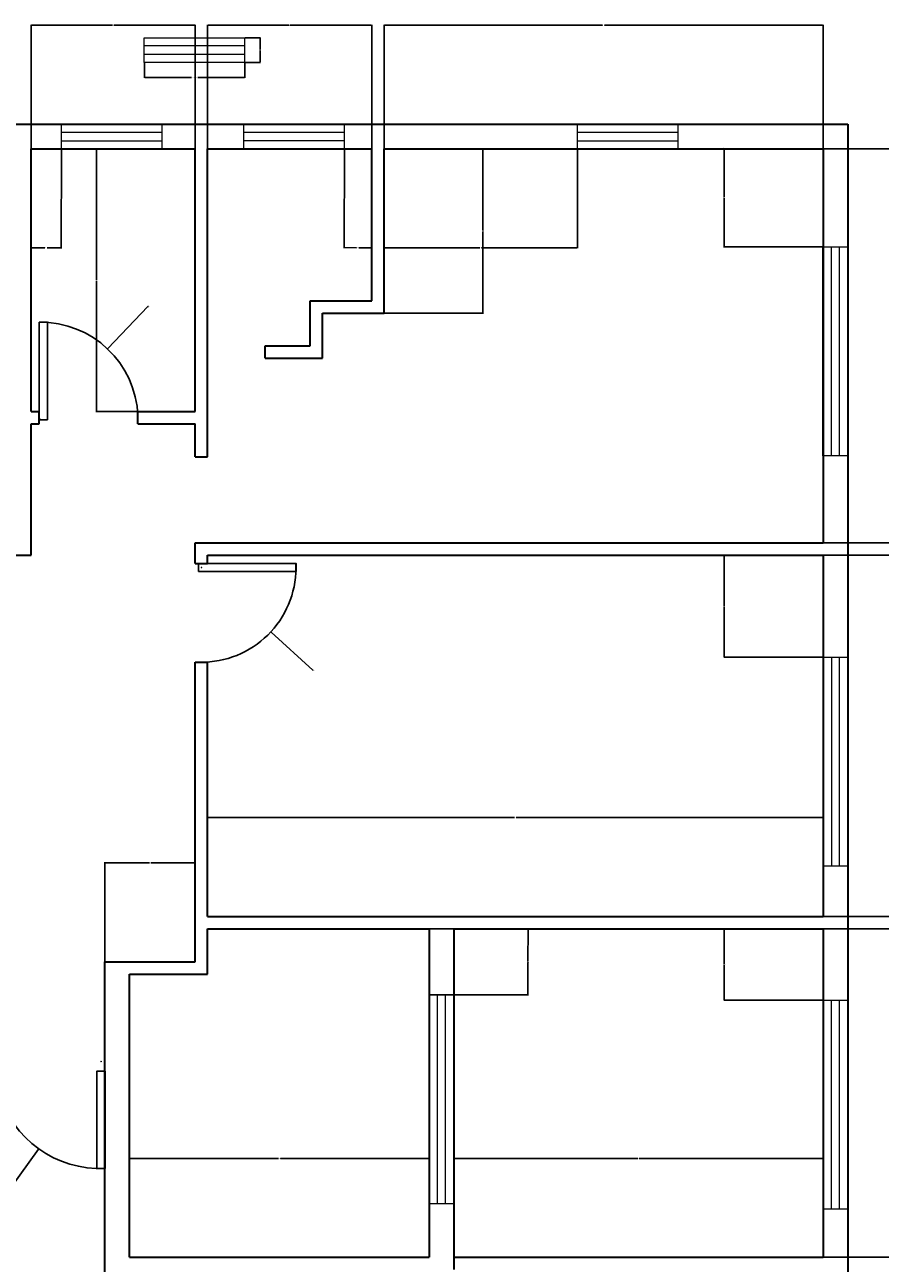
# Model space of a CAD drawing. Units: inches. Extents: x -52 to 1967, y 32 to 824.
# Tile 3 of 10: x 402 to 715, y 372 to 824. Entities that reach past the tile are written whole.
import ezdxf

# ---------------------------------------------------------------- set-up
doc = ezdxf.new("R2010")
doc.units = ezdxf.units.IN
for name, color, linetype, lineweight in [('A-ANNO-DIMS', 2, 'Continuous', 18), ('A-DOOR', 3, 'Continuous', 25), ('A-GLAZ', 4, 'Continuous', 18), ('A-WALL', 7, 'Continuous', 35)]:
    doc.layers.add(name, color=color, linetype=linetype, lineweight=lineweight)
doc.styles.get("Standard").update_dxf_attribs({"font": 'arial.ttf'})
doc.dimstyles.get("Standard").update_dxf_attribs({"dimtxt": 0.18, "dimasz": 0.18, "dimexe": 0.18, "dimexo": 0.0625, "dimgap": 0.09, "dimtad": 0, "dimtih": 1, "dimtoh": 1, "dimdec": 4, "dimzin": 0, "dimdsep": 46, "dimtxsty": 'Standard', "dimcen": 0.09, "dimadec": 0, "dimazin": 0, "dimtfac": 1, "dimtdec": 4, "dimtofl": 0, "dimtmove": 0, "dimatfit": 3, "dimfxl": 1, "dimtolj": 1, "dimtzin": 0, "dimarcsym": 0})

# ---------------------------------------------------------------- blocks, each defined once
blk = doc.blocks.new('WIN-WIDE-76IN')
for p, q in [((0, 0), (0, 9)), ((0, 9), (76.34, 9)), ((76.34, 6), (0, 6)), ((76.34, 9), (76.34, 0)), ((0, 3), (76.34, 3)), ((76.34, 0), (0, 0))]:
    blk.add_line(p, q)
blk = doc.blocks.new('WIN-NARROW-37IN')
for p, q in [((0, 0), (0, 9)), ((0, 9), (36.78, 9)), ((36.78, 6), (0, 6)), ((36.78, 0), (36.78, 9)), ((0, 3), (36.78, 3)), ((36.78, 0), (0, 0))]:
    blk.add_line(p, q)
blk = doc.blocks.new('DOOR-LEAF-36IN')
blk.add_lwpolyline([(0, 0), (-2.98, 0), (-2.98, 35.63), (0, 35.63)], close=True)
blk = doc.blocks.new('*D23')
at = {"layer": 'A-ANNO-DIMS', "color": 0, "lineweight": -2, "transparency": 16777216}
for p, q in [((445.91, 810.52), (445.91, 804.88)), ((482.69, 810.52), (482.69, 804.88)), ((446.09, 805.06), (463.18, 805.06)), ((482.51, 805.06), (465.42, 805.06))]:
    blk.add_line(p, q, dxfattribs=at)
at = {"layer": 'A-ANNO-DIMS', "color": 0, "transparency": 16777216}
for points in [[(446.09, 805.09), (446.09, 805.03), (445.91, 805.06)], [(482.51, 805.09), (482.51, 805.03), (482.69, 805.06)]]:
    blk.add_solid(points, dxfattribs=at)
at = {"layer": 'Defpoints', "color": 0, "transparency": 16777216}
for p in [(445.91, 810.58), (482.69, 810.58), (482.69, 805.06)]:
    blk.add_point(p, dxfattribs=at)
at = {"layer": 'A-ANNO-DIMS', "color": 0, "transparency": 16777216, "insert": (464.3, 805.06), "char_height": 0.18, "attachment_point": 5}
blk.add_mtext('\\A1;WINDOW 37 TYP.', dxfattribs=at)
blk = doc.blocks.new('*D24')
at = {"layer": 'A-ANNO-DIMS', "color": 0, "lineweight": -2, "transparency": 16777216}
for p, q in [((482.75, 819.58), (488.39, 819.58)), ((488.21, 819.4), (488.21, 815.26)), ((488.21, 810.76), (488.21, 814.9)), ((482.75, 810.58), (488.39, 810.58))]:
    blk.add_line(p, q, dxfattribs=at)
at = {"layer": 'A-ANNO-DIMS', "color": 0, "transparency": 16777216}
for points in [[(488.18, 819.4), (488.24, 819.4), (488.21, 819.58)], [(488.18, 810.76), (488.24, 810.76), (488.21, 810.58)]]:
    blk.add_solid(points, dxfattribs=at)
at = {"layer": 'Defpoints', "color": 0, "transparency": 16777216}
for p in [(482.69, 819.58), (488.21, 819.58), (482.69, 810.58)]:
    blk.add_point(p, dxfattribs=at)
at = {"layer": 'A-ANNO-DIMS', "color": 0, "transparency": 16777216, "insert": (488.21, 815.08), "char_height": 0.18, "attachment_point": 5}
blk.add_mtext('\\A1;9 TYP.', dxfattribs=at)
blk = doc.blocks.new('*D56')
at = {"layer": 'A-ANNO-DIMS', "color": 0, "lineweight": -2, "transparency": 16777216}
for p, q in [((404.53, 779.04), (404.53, 824.32)), ((404.71, 824.14), (434.31, 824.14)), ((464.35, 824.14), (434.75, 824.14)), ((464.53, 779.04), (464.53, 824.32))]:
    blk.add_line(p, q, dxfattribs=at)
at = {"layer": 'A-ANNO-DIMS', "color": 0, "transparency": 16777216}
for points in [[(404.71, 824.17), (404.71, 824.11), (404.53, 824.14)], [(464.35, 824.17), (464.35, 824.11), (464.53, 824.14)]]:
    blk.add_solid(points, dxfattribs=at)
at = {"layer": 'Defpoints', "color": 0, "transparency": 16777216}
for p in [(464.53, 824.14), (404.53, 778.97), (464.53, 778.97)]:
    blk.add_point(p, dxfattribs=at)
at = {"layer": 'A-ANNO-DIMS', "color": 0, "transparency": 16777216, "insert": (434.53, 824.14), "char_height": 0.18, "attachment_point": 5}
blk.add_mtext('\\A1;60', dxfattribs=at)
blk = doc.blocks.new('*D57')
at = {"layer": 'A-ANNO-DIMS', "color": 0, "lineweight": -2, "transparency": 16777216}
for p, q in [((469.03, 779.04), (469.03, 824.32)), ((469.21, 824.14), (498.81, 824.14)), ((528.85, 824.14), (499.25, 824.14)), ((529.03, 779.04), (529.03, 824.32))]:
    blk.add_line(p, q, dxfattribs=at)
at = {"layer": 'A-ANNO-DIMS', "color": 0, "transparency": 16777216}
for points in [[(469.21, 824.17), (469.21, 824.11), (469.03, 824.14)], [(528.85, 824.17), (528.85, 824.11), (529.03, 824.14)]]:
    blk.add_solid(points, dxfattribs=at)
at = {"layer": 'Defpoints', "color": 0, "transparency": 16777216}
for p in [(529.03, 824.14), (469.03, 778.97), (529.03, 778.97)]:
    blk.add_point(p, dxfattribs=at)
at = {"layer": 'A-ANNO-DIMS', "color": 0, "transparency": 16777216, "insert": (499.03, 824.14), "char_height": 0.18, "attachment_point": 5}
blk.add_mtext('\\A1;60', dxfattribs=at)
blk = doc.blocks.new('*D58')
at = {"layer": 'A-ANNO-DIMS', "color": 0, "lineweight": -2, "transparency": 16777216}
for p, q in [((533.53, 779.04), (533.53, 824.32)), ((533.71, 824.14), (613.39, 824.14)), ((693.85, 824.14), (614.16, 824.14)), ((694.03, 779.04), (694.03, 824.32))]:
    blk.add_line(p, q, dxfattribs=at)
at = {"layer": 'A-ANNO-DIMS', "color": 0, "transparency": 16777216}
for points in [[(533.71, 824.17), (533.71, 824.11), (533.53, 824.14)], [(693.85, 824.17), (693.85, 824.11), (694.03, 824.14)]]:
    blk.add_solid(points, dxfattribs=at)
at = {"layer": 'Defpoints', "color": 0, "transparency": 16777216}
for p in [(694.03, 824.14), (533.53, 778.97), (694.03, 778.97)]:
    blk.add_point(p, dxfattribs=at)
at = {"layer": 'A-ANNO-DIMS', "color": 0, "transparency": 16777216, "insert": (613.78, 824.14), "char_height": 0.18, "attachment_point": 5}
blk.add_mtext('\\A1;160.5', dxfattribs=at)
blk = doc.blocks.new('*D63')
at = {"layer": 'A-ANNO-DIMS', "color": 0, "lineweight": -2, "transparency": 16777216}
for p, q in [((694.09, 778.97), (739.35, 778.97)), ((739.17, 778.79), (739.17, 707.15)), ((739.17, 635.15), (739.17, 706.79)), ((694.09, 634.97), (739.35, 634.97))]:
    blk.add_line(p, q, dxfattribs=at)
at = {"layer": 'A-ANNO-DIMS', "color": 0, "transparency": 16777216}
for points in [[(739.14, 778.79), (739.2, 778.79), (739.17, 778.97)], [(739.14, 635.15), (739.2, 635.15), (739.17, 634.97)]]:
    blk.add_solid(points, dxfattribs=at)
at = {"layer": 'Defpoints', "color": 0, "transparency": 16777216}
for p in [(694.03, 778.97), (739.17, 778.97), (694.03, 634.97)]:
    blk.add_point(p, dxfattribs=at)
at = {"layer": 'A-ANNO-DIMS', "color": 0, "transparency": 16777216, "insert": (739.17, 706.97), "char_height": 0.18, "attachment_point": 5}
blk.add_mtext('\\A1;144', dxfattribs=at)
blk = doc.blocks.new('*D64')
at = {"layer": 'A-ANNO-DIMS', "color": 0, "lineweight": -2, "transparency": 16777216}
for p, q in [((694.09, 630.47), (739.35, 630.47)), ((739.17, 630.29), (739.17, 564.66)), ((739.17, 498.65), (739.17, 564.29)), ((694.09, 498.47), (739.35, 498.47))]:
    blk.add_line(p, q, dxfattribs=at)
at = {"layer": 'A-ANNO-DIMS', "color": 0, "transparency": 16777216}
for points in [[(739.14, 630.29), (739.2, 630.29), (739.17, 630.47)], [(739.14, 498.65), (739.2, 498.65), (739.17, 498.47)]]:
    blk.add_solid(points, dxfattribs=at)
at = {"layer": 'Defpoints', "color": 0, "transparency": 16777216}
for p in [(694.03, 630.47), (739.17, 630.47), (694.03, 498.47)]:
    blk.add_point(p, dxfattribs=at)
at = {"layer": 'A-ANNO-DIMS', "color": 0, "transparency": 16777216, "insert": (739.17, 564.47), "char_height": 0.18, "attachment_point": 5}
blk.add_mtext('\\A1;132', dxfattribs=at)
blk = doc.blocks.new('*D65')
at = {"layer": 'A-ANNO-DIMS', "color": 0, "lineweight": -2, "transparency": 16777216}
for p, q in [((559.03, 374.04), (559.03, 410.28)), ((559.21, 410.1), (626.25, 410.1)), ((693.85, 410.1), (626.81, 410.1)), ((694.03, 374.04), (694.03, 410.28))]:
    blk.add_line(p, q, dxfattribs=at)
at = {"layer": 'A-ANNO-DIMS', "color": 0, "transparency": 16777216}
for points in [[(559.21, 410.13), (559.21, 410.07), (559.03, 410.1)], [(693.85, 410.13), (693.85, 410.07), (694.03, 410.1)]]:
    blk.add_solid(points, dxfattribs=at)
at = {"layer": 'Defpoints', "color": 0, "transparency": 16777216}
for p in [(694.03, 410.1), (559.03, 373.97), (694.03, 373.97)]:
    blk.add_point(p, dxfattribs=at)
at = {"layer": 'A-ANNO-DIMS', "color": 0, "transparency": 16777216, "insert": (626.53, 410.1), "char_height": 0.18, "attachment_point": 5}
blk.add_mtext('\\A1;135', dxfattribs=at)
blk = doc.blocks.new('*D66')
at = {"layer": 'A-ANNO-DIMS', "color": 0, "lineweight": -2, "transparency": 16777216}
for p, q in [((694.09, 493.97), (739.35, 493.97)), ((739.17, 493.79), (739.17, 434.16)), ((739.17, 374.15), (739.17, 433.79)), ((694.09, 373.97), (739.35, 373.97))]:
    blk.add_line(p, q, dxfattribs=at)
at = {"layer": 'A-ANNO-DIMS', "color": 0, "transparency": 16777216}
for points in [[(739.14, 493.79), (739.2, 493.79), (739.17, 493.97)], [(739.14, 374.15), (739.2, 374.15), (739.17, 373.97)]]:
    blk.add_solid(points, dxfattribs=at)
at = {"layer": 'Defpoints', "color": 0, "transparency": 16777216}
for p in [(694.03, 493.97), (739.17, 493.97), (694.03, 373.97)]:
    blk.add_point(p, dxfattribs=at)
at = {"layer": 'A-ANNO-DIMS', "color": 0, "transparency": 16777216, "insert": (739.17, 433.97), "char_height": 0.18, "attachment_point": 5}
blk.add_mtext('\\A1;120', dxfattribs=at)
blk = doc.blocks.new('*D70')
at = {"layer": 'A-ANNO-DIMS', "color": 0, "lineweight": -2, "transparency": 16777216}
for p, q in [((694.09, 634.97), (739.35, 634.97)), ((739.17, 634.79), (739.17, 632.9)), ((694.09, 630.47), (739.35, 630.47)), ((739.17, 630.65), (739.17, 632.54))]:
    blk.add_line(p, q, dxfattribs=at)
at = {"layer": 'A-ANNO-DIMS', "color": 0, "transparency": 16777216}
for points in [[(739.14, 634.79), (739.2, 634.79), (739.17, 634.97)], [(739.14, 630.65), (739.2, 630.65), (739.17, 630.47)]]:
    blk.add_solid(points, dxfattribs=at)
at = {"layer": 'Defpoints', "color": 0, "transparency": 16777216}
for p in [(694.03, 634.97), (739.17, 634.97), (694.03, 630.47)]:
    blk.add_point(p, dxfattribs=at)
at = {"layer": 'A-ANNO-DIMS', "color": 0, "transparency": 16777216, "insert": (739.17, 632.72), "char_height": 0.18, "attachment_point": 5}
blk.add_mtext('\\A1;4.5', dxfattribs=at)
blk = doc.blocks.new('*D71')
at = {"layer": 'A-ANNO-DIMS', "color": 0, "lineweight": -2, "transparency": 16777216}
for p, q in [((469.03, 498.54), (469.03, 534.78)), ((469.21, 534.6), (581.24, 534.6)), ((693.85, 534.6), (581.82, 534.6)), ((694.03, 498.54), (694.03, 534.78))]:
    blk.add_line(p, q, dxfattribs=at)
at = {"layer": 'A-ANNO-DIMS', "color": 0, "transparency": 16777216}
for points in [[(469.21, 534.63), (469.21, 534.57), (469.03, 534.6)], [(693.85, 534.63), (693.85, 534.57), (694.03, 534.6)]]:
    blk.add_solid(points, dxfattribs=at)
at = {"layer": 'Defpoints', "color": 0, "transparency": 16777216}
for p in [(694.03, 534.6), (469.03, 498.47), (694.03, 498.47)]:
    blk.add_point(p, dxfattribs=at)
at = {"layer": 'A-ANNO-DIMS', "color": 0, "transparency": 16777216, "insert": (581.53, 534.6), "char_height": 0.18, "attachment_point": 5}
blk.add_mtext('\\A1;225', dxfattribs=at)
blk = doc.blocks.new('*D72')
at = {"layer": 'A-ANNO-DIMS', "color": 0, "lineweight": -2, "transparency": 16777216}
for p, q in [((440.53, 374.04), (440.53, 410.28)), ((440.71, 410.1), (494.89, 410.1)), ((549.85, 410.1), (495.66, 410.1)), ((550.03, 374.04), (550.03, 410.28))]:
    blk.add_line(p, q, dxfattribs=at)
at = {"layer": 'A-ANNO-DIMS', "color": 0, "transparency": 16777216}
for points in [[(440.71, 410.13), (440.71, 410.07), (440.53, 410.1)], [(549.85, 410.13), (549.85, 410.07), (550.03, 410.1)]]:
    blk.add_solid(points, dxfattribs=at)
at = {"layer": 'Defpoints', "color": 0, "transparency": 16777216}
for p in [(550.03, 410.1), (440.53, 373.97), (550.03, 373.97)]:
    blk.add_point(p, dxfattribs=at)
at = {"layer": 'A-ANNO-DIMS', "color": 0, "transparency": 16777216, "insert": (495.28, 410.1), "char_height": 0.18, "attachment_point": 5}
blk.add_mtext('\\A1;109.5', dxfattribs=at)
blk = doc.blocks.new('*D76')
at = {"layer": 'A-ANNO-DIMS', "color": 0, "lineweight": -2, "transparency": 16777216}
for p, q in [((404.53, 778.91), (404.38, 742.66)), ((415.69, 778.87), (415.54, 742.62)), ((404.56, 742.84), (409.51, 742.82)), ((415.36, 742.8), (410.42, 742.82))]:
    blk.add_line(p, q, dxfattribs=at)
at = {"layer": 'A-ANNO-DIMS', "color": 0, "transparency": 16777216}
for points in [[(404.56, 742.87), (404.56, 742.81), (404.38, 742.84)], [(415.36, 742.83), (415.36, 742.77), (415.54, 742.8)]]:
    blk.add_solid(points, dxfattribs=at)
at = {"layer": 'Defpoints', "color": 0, "transparency": 16777216}
for p in [(404.53, 778.97), (415.69, 778.93), (404.38, 742.84)]:
    blk.add_point(p, dxfattribs=at)
at = {"layer": 'A-ANNO-DIMS', "color": 0, "transparency": 16777216, "insert": (409.96, 742.82), "char_height": 0.18, "attachment_point": 5}
blk.add_mtext('\\A1;11.165', dxfattribs=at)
blk = doc.blocks.new('*D77')
at = {"layer": 'A-ANNO-DIMS', "color": 0, "lineweight": -2, "transparency": 16777216}
for p, q in [((519.02, 778.95), (518.9, 742.7)), ((529.03, 778.91), (528.9, 742.66)), ((519.08, 742.88), (523.44, 742.86)), ((528.72, 742.84), (524.35, 742.86))]:
    blk.add_line(p, q, dxfattribs=at)
at = {"layer": 'A-ANNO-DIMS', "color": 0, "transparency": 16777216}
for points in [[(519.08, 742.91), (519.08, 742.85), (518.9, 742.88)], [(528.72, 742.87), (528.72, 742.81), (528.9, 742.84)]]:
    blk.add_solid(points, dxfattribs=at)
at = {"layer": 'Defpoints', "color": 0, "transparency": 16777216}
for p in [(519.02, 779.01), (529.03, 778.97), (518.9, 742.88)]:
    blk.add_point(p, dxfattribs=at)
at = {"layer": 'A-ANNO-DIMS', "color": 0, "transparency": 16777216, "insert": (523.9, 742.86), "char_height": 0.18, "attachment_point": 5}
blk.add_mtext('\\A1;10.005', dxfattribs=at)
blk = doc.blocks.new('*D78')
at = {"layer": 'A-ANNO-DIMS', "color": 0, "lineweight": -2, "transparency": 16777216}
for p, q in [((533.53, 778.91), (533.51, 742.66)), ((604.23, 778.88), (604.21, 742.63)), ((533.69, 742.84), (568.54, 742.83)), ((604.03, 742.81), (569.18, 742.83))]:
    blk.add_line(p, q, dxfattribs=at)
at = {"layer": 'A-ANNO-DIMS', "color": 0, "transparency": 16777216}
for points in [[(533.69, 742.87), (533.69, 742.81), (533.51, 742.84)], [(604.03, 742.84), (604.03, 742.78), (604.21, 742.81)]]:
    blk.add_solid(points, dxfattribs=at)
at = {"layer": 'Defpoints', "color": 0, "transparency": 16777216}
for p in [(533.53, 778.97), (604.23, 778.94), (533.51, 742.84)]:
    blk.add_point(p, dxfattribs=at)
at = {"layer": 'A-ANNO-DIMS', "color": 0, "transparency": 16777216, "insert": (568.86, 742.83), "char_height": 0.18, "attachment_point": 5}
blk.add_mtext('\\A1;70.7', dxfattribs=at)
blk = doc.blocks.new('*D80')
at = {"layer": 'A-ANNO-DIMS', "color": 0, "lineweight": -2, "transparency": 16777216}
for p, q in [((533.59, 778.97), (569.84, 778.97)), ((569.66, 778.79), (569.66, 749.16)), ((569.66, 719.15), (569.66, 748.79)), ((533.59, 718.97), (569.84, 718.97))]:
    blk.add_line(p, q, dxfattribs=at)
at = {"layer": 'A-ANNO-DIMS', "color": 0, "transparency": 16777216}
for points in [[(569.63, 778.79), (569.69, 778.79), (569.66, 778.97)], [(569.63, 719.15), (569.69, 719.15), (569.66, 718.97)]]:
    blk.add_solid(points, dxfattribs=at)
at = {"layer": 'Defpoints', "color": 0, "transparency": 16777216}
for p in [(533.53, 778.97), (533.53, 718.97), (569.66, 718.97)]:
    blk.add_point(p, dxfattribs=at)
at = {"layer": 'A-ANNO-DIMS', "color": 0, "transparency": 16777216, "insert": (569.66, 748.97), "char_height": 0.18, "attachment_point": 5}
blk.add_mtext('\\A1;60', dxfattribs=at)
blk = doc.blocks.new('*D81')
at = {"layer": 'A-ANNO-DIMS', "color": 0, "lineweight": -2, "transparency": 16777216}
for p, q in [((464.46, 778.97), (428.22, 778.97)), ((428.4, 778.79), (428.4, 731.16)), ((428.4, 683.15), (428.4, 730.79)), ((464.46, 682.97), (428.22, 682.97))]:
    blk.add_line(p, q, dxfattribs=at)
at = {"layer": 'A-ANNO-DIMS', "color": 0, "transparency": 16777216}
for points in [[(428.37, 778.79), (428.43, 778.79), (428.4, 778.97)], [(428.37, 683.15), (428.43, 683.15), (428.4, 682.97)]]:
    blk.add_solid(points, dxfattribs=at)
at = {"layer": 'Defpoints', "color": 0, "transparency": 16777216}
for p in [(428.4, 778.97), (464.53, 778.97), (464.53, 682.97)]:
    blk.add_point(p, dxfattribs=at)
at = {"layer": 'A-ANNO-DIMS', "color": 0, "transparency": 16777216, "insert": (428.4, 730.97), "char_height": 0.18, "attachment_point": 5}
blk.add_mtext('\\A1;96', dxfattribs=at)
blk = doc.blocks.new('*D82')
at = {"layer": 'A-ANNO-DIMS', "color": 0, "lineweight": -2, "transparency": 16777216}
for p, q in [((693.96, 778.97), (657.72, 779.05)), ((657.9, 778.87), (657.86, 761.31)), ((657.82, 743.39), (657.86, 760.94)), ((693.89, 743.13), (657.64, 743.21))]:
    blk.add_line(p, q, dxfattribs=at)
at = {"layer": 'A-ANNO-DIMS', "color": 0, "transparency": 16777216}
for points in [[(657.87, 778.87), (657.93, 778.87), (657.9, 779.05)], [(657.79, 743.39), (657.85, 743.39), (657.82, 743.21)]]:
    blk.add_solid(points, dxfattribs=at)
at = {"layer": 'Defpoints', "color": 0, "transparency": 16777216}
for p in [(657.9, 779.05), (694.03, 778.97), (693.95, 743.13)]:
    blk.add_point(p, dxfattribs=at)
at = {"layer": 'A-ANNO-DIMS', "color": 0, "transparency": 16777216, "insert": (657.86, 761.13), "char_height": 0.18, "attachment_point": 5}
blk.add_mtext('\\A1;35.84', dxfattribs=at)
blk = doc.blocks.new('*D83')
at = {"layer": 'A-ANNO-DIMS', "color": 0, "lineweight": -2, "transparency": 16777216}
for p, q in [((693.96, 630.47), (657.72, 630.46)), ((657.9, 630.28), (657.9, 612.01)), ((657.91, 593.38), (657.9, 611.65)), ((693.98, 593.22), (657.73, 593.2))]:
    blk.add_line(p, q, dxfattribs=at)
at = {"layer": 'A-ANNO-DIMS', "color": 0, "transparency": 16777216}
for points in [[(657.93, 630.28), (657.87, 630.28), (657.9, 630.46)], [(657.94, 593.38), (657.88, 593.38), (657.91, 593.2)]]:
    blk.add_solid(points, dxfattribs=at)
at = {"layer": 'Defpoints', "color": 0, "transparency": 16777216}
for p in [(657.9, 630.46), (694.03, 630.47), (694.04, 593.22)]:
    blk.add_point(p, dxfattribs=at)
at = {"layer": 'A-ANNO-DIMS', "color": 0, "transparency": 16777216, "insert": (657.9, 611.83), "char_height": 0.18, "attachment_point": 5}
blk.add_mtext('\\A1;37.254', dxfattribs=at)
blk = doc.blocks.new('*D84')
at = {"layer": 'A-ANNO-DIMS', "color": 0, "lineweight": -2, "transparency": 16777216}
for p, q in [((693.96, 493.97), (657.72, 493.98)), ((657.9, 493.8), (657.89, 481.12)), ((657.89, 468.07), (657.89, 480.76)), ((693.96, 467.88), (657.71, 467.89))]:
    blk.add_line(p, q, dxfattribs=at)
at = {"layer": 'A-ANNO-DIMS', "color": 0, "transparency": 16777216}
for points in [[(657.87, 493.8), (657.93, 493.8), (657.9, 493.98)], [(657.86, 468.07), (657.92, 468.07), (657.89, 467.89)]]:
    blk.add_solid(points, dxfattribs=at)
at = {"layer": 'Defpoints', "color": 0, "transparency": 16777216}
for p in [(657.9, 493.98), (694.03, 493.97), (694.02, 467.88)]:
    blk.add_point(p, dxfattribs=at)
at = {"layer": 'A-ANNO-DIMS', "color": 0, "transparency": 16777216, "insert": (657.89, 480.94), "char_height": 0.18, "attachment_point": 5}
blk.add_mtext('\\A1;26.094', dxfattribs=at)
blk = doc.blocks.new('*D86')
at = {"layer": 'A-ANNO-DIMS', "color": 0, "lineweight": -2, "transparency": 16777216}
for p, q in [((550.09, 493.97), (586.34, 493.92)), ((586.16, 493.74), (586.14, 482.05)), ((586.12, 469.99), (586.14, 481.68)), ((550.06, 469.86), (586.3, 469.81))]:
    blk.add_line(p, q, dxfattribs=at)
at = {"layer": 'A-ANNO-DIMS', "color": 0, "transparency": 16777216}
for points in [[(586.13, 493.74), (586.19, 493.74), (586.16, 493.92)], [(586.09, 469.99), (586.15, 469.99), (586.12, 469.81)]]:
    blk.add_solid(points, dxfattribs=at)
at = {"layer": 'Defpoints', "color": 0, "transparency": 16777216}
for p in [(550.03, 493.97), (549.99, 469.86), (586.12, 469.81)]:
    blk.add_point(p, dxfattribs=at)
at = {"layer": 'A-ANNO-DIMS', "color": 0, "transparency": 16777216, "insert": (586.14, 481.87), "char_height": 0.18, "attachment_point": 5}
blk.add_mtext('\\A1;24.115', dxfattribs=at)
blk = doc.blocks.new('*D89')
at = {"layer": 'A-ANNO-DIMS', "color": 0, "lineweight": -2, "transparency": 16777216}
for p, q in [((431.53, 482.04), (431.53, 518.28)), ((431.71, 518.1), (447.81, 518.1)), ((464.35, 518.1), (448.25, 518.1)), ((464.53, 482.04), (464.53, 518.28))]:
    blk.add_line(p, q, dxfattribs=at)
at = {"layer": 'A-ANNO-DIMS', "color": 0, "transparency": 16777216}
for points in [[(431.71, 518.13), (431.71, 518.07), (431.53, 518.1)], [(464.35, 518.13), (464.35, 518.07), (464.53, 518.1)]]:
    blk.add_solid(points, dxfattribs=at)
at = {"layer": 'Defpoints', "color": 0, "transparency": 16777216}
for p in [(464.53, 518.1), (431.53, 481.97), (464.53, 481.97)]:
    blk.add_point(p, dxfattribs=at)
at = {"layer": 'A-ANNO-DIMS', "color": 0, "transparency": 16777216, "insert": (448.03, 518.1), "char_height": 0.18, "attachment_point": 5}
blk.add_mtext('\\A1;33', dxfattribs=at)
blk = doc.blocks.new('*D135')
at = {"layer": 'A-ANNO-DIMS', "color": 0, "lineweight": -2, "transparency": 16777216}
for p, q in [((430, 445.49), (430.18, 445.49)), ((430.09, 445.4), (430.09, 445.58)), ((393.63, 394.5), (407.2, 413.48)), ((393.45, 394.5), (393.63, 394.5))]:
    blk.add_line(p, q, dxfattribs=at)
at = {"layer": 'A-ANNO-DIMS', "color": 0, "transparency": 16777216}
blk.add_solid([(407.18, 413.49), (407.22, 413.46), (407.3, 413.62)], dxfattribs=at)
at = {"layer": 'Defpoints', "color": 0, "transparency": 16777216}
for p in [(430.09, 445.49), (407.3, 413.62)]:
    blk.add_point(p, dxfattribs=at)
at = {"layer": 'A-ANNO-DIMS', "color": 0, "transparency": 16777216, "insert": (392.97, 394.5), "char_height": 0.18, "attachment_point": 5}
blk.add_mtext('\\A1;R39.17', dxfattribs=at)
blk = doc.blocks.new('*D137')
at = {"layer": 'A-ANNO-DIMS', "color": 0, "lineweight": -2, "transparency": 16777216}
for p, q in [((447.22, 721.32), (432.62, 705.97)), ((447.4, 721.32), (447.22, 721.32)), ((407.88, 680.04), (408.06, 680.04)), ((407.97, 679.95), (407.97, 680.13))]:
    blk.add_line(p, q, dxfattribs=at)
at = {"layer": 'A-ANNO-DIMS', "color": 0, "transparency": 16777216}
blk.add_solid([(432.6, 705.99), (432.64, 705.95), (432.5, 705.84)], dxfattribs=at)
at = {"layer": 'Defpoints', "color": 0, "transparency": 16777216}
for p in [(432.5, 705.84), (407.97, 680.04)]:
    blk.add_point(p, dxfattribs=at)
at = {"layer": 'A-ANNO-DIMS', "color": 0, "transparency": 16777216, "insert": (447.8, 721.32), "char_height": 0.18, "attachment_point": 5}
blk.add_mtext('\\A1;R35.6', dxfattribs=at)
blk = doc.blocks.new('*D138')
at = {"layer": 'A-ANNO-DIMS', "color": 0, "lineweight": -2, "transparency": 16777216}
for p, q in [((466.71, 625.95), (466.89, 625.95)), ((466.8, 625.86), (466.8, 626.04)), ((507.44, 588.49), (492.33, 602.42)), ((507.62, 588.49), (507.44, 588.49))]:
    blk.add_line(p, q, dxfattribs=at)
at = {"layer": 'A-ANNO-DIMS', "color": 0, "transparency": 16777216}
blk.add_solid([(492.35, 602.44), (492.31, 602.39), (492.2, 602.54)], dxfattribs=at)
at = {"layer": 'Defpoints', "color": 0, "transparency": 16777216}
for p in [(466.8, 625.95), (492.2, 602.54)]:
    blk.add_point(p, dxfattribs=at)
at = {"layer": 'A-ANNO-DIMS', "color": 0, "transparency": 16777216, "insert": (508.1, 588.49), "char_height": 0.18, "attachment_point": 5}
blk.add_mtext('\\A1;R34.55', dxfattribs=at)

msp = doc.modelspace()

# ---------------------------------------------------------------- linework, layer by layer
at = {"layer": 'A-DOOR'}
for centre, radius, start, end in [((407.9722, 680.042), 35.597, 2.062429, 90.834349), ((466.7999, 625.9527), 34.5471, 272.178706, 2.484769), ((430.0876, 445.4886), 39.1725, 196.688789, 272.182514)]:
    msp.add_arc(centre, radius, start, end, dxfattribs=at)
at = {"layer": 'A-WALL'}
for p, q in [((223.0273, 787.9731), (703.0273, 787.9731)), ((703.0273, 787.9731), (703.0273, 67.9731)), ((404.5273, 778.9731), (464.5273, 778.9731)), ((404.5273, 682.9731), (404.5273, 778.9731)), ((464.5273, 682.9731), (464.5273, 778.9731)), ((469.0273, 778.9731), (529.0273, 778.9731)), ((469.0273, 666.4731), (469.0273, 778.9731)), ((529.0273, 723.4731), (529.0273, 778.9731)), ((533.5273, 718.9731), (533.5273, 778.9731)), ((533.5273, 778.9731), (694.0273, 778.9731)), ((694.0273, 778.9731), (694.0273, 634.9731)), ((506.5273, 706.9731), (506.5273, 723.4731)), ((506.5273, 723.4731), (529.0273, 723.4731)), ((511.0273, 702.4731), (511.0273, 718.9731)), ((511.0273, 718.9731), (533.5273, 718.9731)), ((490.0273, 706.9731), (506.5273, 706.9731)), ((490.0273, 702.4731), (490.0273, 706.9731)), ((490.0273, 702.4731), (511.0273, 702.4731)), ((404.5273, 682.9731), (407.5273, 682.9731)), ((407.5273, 678.4731), (407.5273, 682.9731)), ((443.5273, 682.9731), (464.5273, 682.9731)), ((443.5273, 678.4731), (443.5273, 682.9731)), ((404.5273, 630.4731), (404.5273, 678.4731)), ((404.5273, 678.4731), (407.5273, 678.4731)), ((443.5273, 678.4731), (464.5273, 678.4731)), ((464.5273, 666.4731), (464.5273, 678.4731)), ((464.5273, 666.4731), (469.0273, 666.4731)), ((464.5273, 630.4731), (464.5273, 634.9731)), ((464.5273, 634.9731), (694.0273, 634.9731)), ((464.5273, 627.4731), (464.5273, 634.9731)), ((232.0273, 630.4731), (404.5273, 630.4731)), ((469.0273, 630.4731), (694.0273, 630.4731)), ((469.0273, 627.4731), (469.0273, 630.4731)), ((694.0273, 630.4731), (694.0273, 498.4731)), ((464.5273, 627.4731), (469.0273, 627.4731)), ((464.5273, 481.9731), (464.5273, 591.4731)), ((464.5273, 591.4731), (469.0273, 591.4731)), ((469.0273, 498.4731), (469.0273, 591.4731)), ((469.0273, 498.4731), (694.0273, 498.4731)), ((469.0273, 493.9731), (550.0273, 493.9731)), ((469.0273, 477.4731), (469.0273, 493.9731)), ((550.0273, 493.9731), (550.0273, 373.9731)), ((559.0273, 493.9731), (559.0273, 369.4731)), ((559.0273, 493.9731), (694.0273, 493.9731)), ((694.0273, 493.9731), (694.0273, 373.9731)), ((431.5273, 481.9731), (464.5273, 481.9731)), ((431.5273, 360.4731), (431.5273, 481.9731)), ((440.5273, 477.4731), (469.0273, 477.4731)), ((440.5273, 373.9731), (440.5273, 477.4731)), ((440.5273, 373.9731), (550.0273, 373.9731)), ((559.0273, 373.9731), (694.0273, 373.9731))]:
    msp.add_line(p, q, dxfattribs=at)

# ---------------------------------------------------------------- block references
at = {"layer": 'A-DOOR'}
for p in [(410.4815, 679.9838), (431.5768, 406.3464)]:
    msp.add_blockref('DOOR-LEAF-36IN', p, dxfattribs=at)
at = {"layer": 'A-DOOR', "rotation": 269.9999999999995}
msp.add_blockref('DOOR-LEAF-36IN', (465.7286, 624.4977), dxfattribs=at)
at = {"layer": 'A-GLAZ'}
for p in [(445.9093, 810.5819), (415.6918, 778.9277), (482.2409, 779.008), (604.2269, 778.942)]:
    msp.add_blockref('WIN-NARROW-37IN', p, dxfattribs=at)
for p, rotation in [((693.9542, 743.1315), 270), ((694.0428, 593.2193), 269.9999999999998), ((549.994, 469.8581), 270), ((694.0191, 467.8793), 270)]:
    msp.add_blockref('WIN-WIDE-76IN', p, dxfattribs=dict(at, rotation=rotation))

# ---------------------------------------------------------------- dimensions: what is measured, and where the dimension line sits
at = {"layer": 'A-ANNO-DIMS'}
for base, p1, p2, override, picture, middle in [((464.5273, 824.138), (404.5273, 778.9731), (464.5273, 778.9731), {"dimdec": 0, "dimlfac": 1, "dimrnd": 0, "dimzin": 0, "dimdsep": 46, "dimlunit": 2}, '*D56', (434.5273, 824.138)), ((529.0273, 824.138), (469.0273, 778.9731), (529.0273, 778.9731), {"dimdec": 0, "dimlfac": 1, "dimrnd": 0, "dimzin": 0, "dimdsep": 46, "dimlunit": 2}, '*D57', (499.0273, 824.138)), ((694.0273, 824.138), (533.5273, 778.9731), (694.0273, 778.9731), {"dimdec": 1, "dimlfac": 1, "dimrnd": 0, "dimzin": 0, "dimdsep": 46, "dimlunit": 2}, '*D58', (613.7773, 824.138)), ((694.0273, 534.6031), (469.0273, 498.4731), (694.0273, 498.4731), {"dimdec": 0, "dimlfac": 1, "dimrnd": 0, "dimzin": 0, "dimdsep": 46, "dimlunit": 2}, '*D71', (581.5273, 534.6031)), ((464.5273, 518.1031), (431.5273, 481.9731), (464.5273, 481.9731), {"dimdec": 0, "dimlfac": 1, "dimrnd": 0, "dimzin": 0, "dimdsep": 46, "dimlunit": 2}, '*D89', (448.0273, 518.1031)), ((550.0273, 410.1031), (440.5273, 373.9731), (550.0273, 373.9731), {"dimdec": 1, "dimlfac": 1, "dimrnd": 0, "dimzin": 0, "dimdsep": 46, "dimlunit": 2}, '*D72', (495.2773, 410.1031)), ((694.0273, 410.1031), (559.0273, 373.9731), (694.0273, 373.9731), {"dimdec": 0, "dimlfac": 1, "dimrnd": 0, "dimzin": 0, "dimdsep": 46, "dimlunit": 2}, '*D65', (626.5273, 410.1031))]:
    dim = msp.add_linear_dim(base=base, p1=p1, p2=p2, dimstyle='Standard', override=override, dxfattribs=at)
    dim.commit()
    dim.dimension.update_dxf_attribs({"geometry": picture, "text_midpoint": middle})
dim = msp.add_linear_dim(base=(488.2082, 819.5819), p1=(482.6909, 810.5819), p2=(482.6909, 819.5819), angle=90, text='<> TYP.', dimstyle='Standard', override={"dimdec": 0, "dimlfac": 1, "dimrnd": 0, "dimzin": 0, "dimdsep": 46, "dimlunit": 2}, dxfattribs=at)
dim.commit()
dim.dimension.update_dxf_attribs({"geometry": '*D24', "text_midpoint": (488.2082, 815.0819)})
dim = msp.add_linear_dim(base=(482.6909, 805.0646), p1=(445.9093, 810.5819), p2=(482.6909, 810.5819), text='WINDOW <> TYP.', dimstyle='Standard', override={"dimdec": 0, "dimlfac": 1, "dimrnd": 0, "dimzin": 0, "dimdsep": 46, "dimlunit": 2}, dxfattribs=at)
dim.commit()
dim.dimension.update_dxf_attribs({"geometry": '*D23', "text_midpoint": (464.3001, 805.0646)})
for base, p1, p2, angle, override, picture, middle in [((404.3801, 742.8434), (415.6918, 778.9277), (404.5273, 778.9731), 179.766633, {"dimdec": 3, "dimlfac": 1, "dimrnd": 0, "dimzin": 0, "dimdsep": 46, "dimlunit": 2}, '*D76', (409.9624, 742.8207)), ((428.3973, 778.9731), (464.5273, 682.9731), (464.5273, 778.9731), 90, {"dimdec": 0, "dimlfac": 1, "dimrnd": 0, "dimzin": 0, "dimdsep": 46, "dimlunit": 2}, '*D81', (428.3973, 730.9731)), ((518.8967, 742.8782), (529.0273, 778.9731), (519.0226, 779.008), 179.800394, {"dimdec": 3, "dimlfac": 1, "dimrnd": 0, "dimzin": 0, "dimdsep": 46, "dimlunit": 2}, '*D77', (523.8991, 742.8608)), ((533.5113, 742.8431), (604.2269, 778.942), (533.5273, 778.9731), 179.974743, {"dimdec": 1, "dimlfac": 1, "dimrnd": 0, "dimzin": 0, "dimdsep": 46, "dimlunit": 2}, '*D78', (568.8612, 742.8276)), ((569.6573, 718.9731), (533.5273, 778.9731), (533.5273, 718.9731), 270, {"dimdec": 0, "dimlfac": 1, "dimrnd": 0, "dimzin": 0, "dimdsep": 46, "dimlunit": 2}, '*D80', (569.6573, 748.9731)), ((657.8973, 779.0468), (693.9542, 743.1315), (694.0273, 778.9731), 89.88322, {"dimdec": 2, "dimlfac": 1, "dimrnd": 0, "dimzin": 0, "dimdsep": 46, "dimlunit": 2}, '*D82', (657.8608, 761.1259)), ((739.1728, 778.9731), (694.0273, 634.9731), (694.0273, 778.9731), 90, {"dimdec": 0, "dimlfac": 1, "dimrnd": 0, "dimzin": 0, "dimdsep": 46, "dimlunit": 2}, '*D63', (739.1728, 706.9731)), ((739.1728, 634.9731), (694.0273, 630.4731), (694.0273, 634.9731), 90, {"dimdec": 1, "dimlfac": 1, "dimrnd": 0, "dimzin": 0, "dimdsep": 46, "dimlunit": 2}, '*D70', (739.1728, 632.7231)), ((657.8973, 630.4581), (694.0428, 593.2193), (694.0273, 630.4731), 90.023836, {"dimdec": 3, "dimlfac": 1, "dimrnd": 0, "dimzin": 0, "dimdsep": 46, "dimlunit": 2}, '*D83', (657.905, 611.8312)), ((739.1728, 630.4731), (694.0273, 498.4731), (694.0273, 630.4731), 90, {"dimdec": 0, "dimlfac": 1, "dimrnd": 0, "dimzin": 0, "dimdsep": 46, "dimlunit": 2}, '*D64', (739.1728, 564.4731)), ((586.124, 469.8083), (550.0273, 493.9731), (549.994, 469.8581), 269.920999, {"dimdec": 3, "dimlfac": 1, "dimrnd": 0, "dimzin": 0, "dimdsep": 46, "dimlunit": 2}, '*D86', (586.1406, 481.8658)), ((657.8973, 493.9844), (694.0191, 467.8793), (694.0273, 493.9731), 89.982145, {"dimdec": 3, "dimlfac": 1, "dimrnd": 0, "dimzin": 0, "dimdsep": 46, "dimlunit": 2}, '*D84', (657.8932, 480.9375)), ((739.1728, 493.9731), (694.0273, 373.9731), (694.0273, 493.9731), 90, {"dimdec": 0, "dimlfac": 1, "dimrnd": 0, "dimzin": 0, "dimdsep": 46, "dimlunit": 2}, '*D66', (739.1728, 433.9731))]:
    dim = msp.add_linear_dim(base=base, p1=p1, p2=p2, angle=angle, dimstyle='Standard', override=override, dxfattribs=at)
    dim.commit()
    dim.dimension.update_dxf_attribs({"geometry": picture, "text_midpoint": middle})
for center, mpoint, override, picture, middle in [((407.9722, 680.042), (432.499, 705.841), {"dimdec": 1, "dimlfac": 1, "dimrnd": 0, "dimzin": 0, "dimdsep": 46, "dimlunit": 2}, '*D137', (447.8049, 721.3203)), ((466.7999, 625.9527), (492.2019, 602.5381), {"dimdec": 2, "dimlfac": 1, "dimrnd": 0, "dimzin": 0, "dimdsep": 46, "dimlunit": 2}, '*D138', (508.1036, 588.4893)), ((430.0876, 445.4886), (407.3042, 413.6232), {"dimdec": 2, "dimlfac": 1, "dimrnd": 0, "dimzin": 0, "dimdsep": 46, "dimlunit": 2}, '*D135', (392.9743, 394.504))]:
    dim = msp.add_radius_dim(center=center, mpoint=mpoint, dimstyle='Standard', override=override, dxfattribs=at)
    dim.commit()
    dim.dimension.update_dxf_attribs({"geometry": picture, "text_midpoint": middle, "dimtype": 164})

doc.saveas('drawing.dxf')
